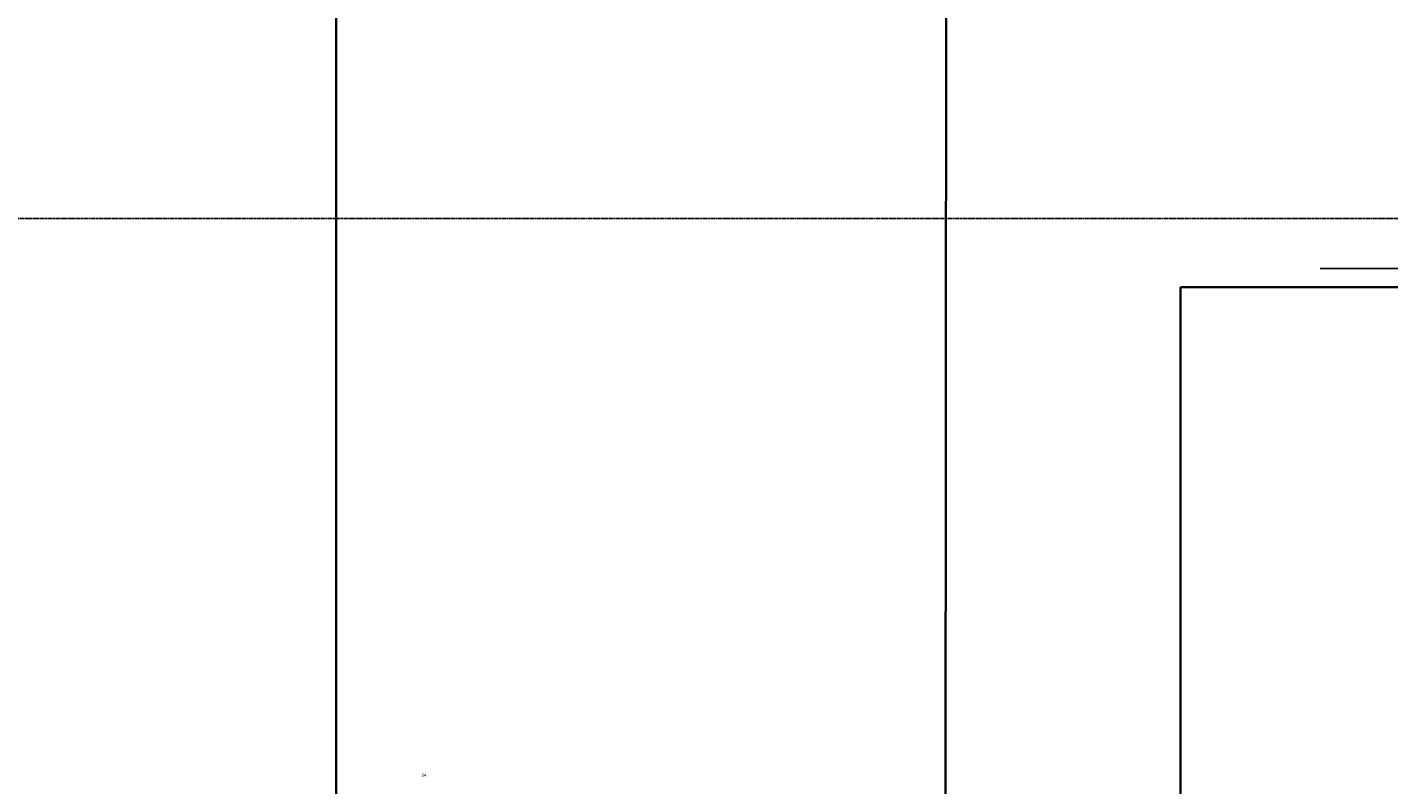
# Model space of a CAD drawing. Units: millimetres. Extents: x 353872 to 441597, y 126154 to 187356.
# Tile 15 of 28: x 391248 to 399262, y 153772 to 158230. Entities that reach past the tile are written whole.
import ezdxf

# ---------------------------------------------------------------- set-up
doc = ezdxf.new("R2010")
doc.units = ezdxf.units.MM
doc.linetypes.add('ACAD_ISO02W100', pattern=[15, 12, -3])
doc.layers.add('AC-UINT', color=2, linetype='Continuous')
for name, color, linetype, lineweight in [('P-ANNO-TEXT', 7, 'Continuous', 25), ('P-BNDY', 4, 'ACAD_ISO02W100', 25), ('P-PIPE', 3, 'Continuous', 35), ('P-PIPE-FITT', 6, 'Continuous', 25)]:
    doc.layers.add(name, color=color, linetype=linetype, lineweight=lineweight)
doc.styles.get("Standard").update_dxf_attribs({"font": 'arial.ttf'})

# ---------------------------------------------------------------- blocks, each defined once
blk = doc.blocks.new('DFSG')
at = {"layer": 'AC-UINT', "ltscale": 3}
blk.add_line((94.3237, -27.1601), (94.091, -27.1601), dxfattribs=at)
blk.add_solid([(94.091, -27.1214), (94.0909, -27.1989), (93.8965, -27.1598)], dxfattribs=at)

msp = doc.modelspace()

# ---------------------------------------------------------------- linework, layer by layer
at = {"layer": 'P-BNDY'}
msp.add_line((436591, 157104.68), (386532.91, 157104.68), dxfattribs=at)
at = {"layer": 'P-PIPE'}
for p, q in [((396659.16, 160948.84), (396648.15, 149319.73)), ((399938.88, 156699.54), (398036.88, 156699.54)), ((398036.88, 156699.54), (398036.88, 150168.41))]:
    msp.add_line(p, q, dxfattribs=at)
msp.add_lwpolyline([(393066.71, 149319.73), (393066.71, 175399.89), (426420.76, 175399.89)], dxfattribs=at)

# ---------------------------------------------------------------- block references
at = {"layer": 'P-PIPE-FITT', "xscale": 2079.990875364621, "yscale": 2079.990875364621, "zscale": 2079.990875364621, "rotation": 179.9589088552121}
msp.add_blockref('DFSG', (595010.25, 100175.78), dxfattribs=at)

# ---------------------------------------------------------------- texts
at = {"layer": 'P-ANNO-TEXT'}
msp.add_text('S4', height=18.55, dxfattribs=at).set_placement((393568.56, 153818.82))

doc.saveas('drawing.dxf')
